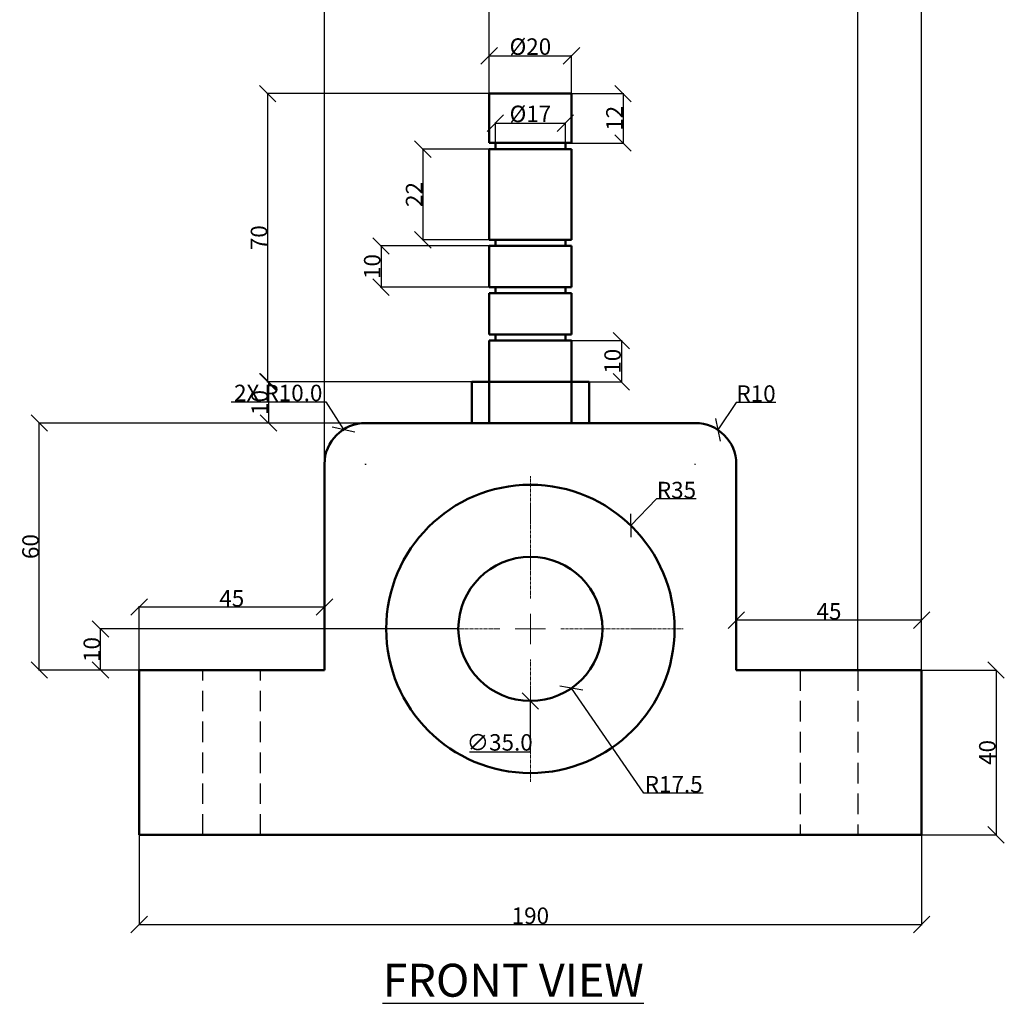
# Model space of a CAD drawing. Units: millimetres. Extents: x 2623 to 3019, y 2308 to 2699.
# Tile 1 of 3: x 2623 to 2862, y 2308 to 2547. Entities that reach past the tile are written whole.
import ezdxf

# ---------------------------------------------------------------- set-up
doc = ezdxf.new("R2010")
doc.units = ezdxf.units.MM
doc.header["$MEASUREMENT"] = 0
doc.linetypes.add('CENTER2', pattern=[1.125, 0.75, -0.125, 0.125, -0.125])
doc.linetypes.add('HIDDEN', pattern=[0.375, 0.25, -0.125])
for name, color, linetype, lineweight in [('M-CNTR', 1, 'CENTER2', 18), ('M-DIMS', 2, 'Continuous', 25), ('M-HIDN', 8, 'HIDDEN', 25), ('M-OUTL', 7, 'Continuous', 50), ('M-TEXT', 7, 'Continuous', 25)]:
    doc.layers.add(name, color=color, linetype=linetype, lineweight=lineweight)
doc.styles.get("Standard").update_dxf_attribs({"font": 'arial.ttf'})
doc.dimstyles.get("Standard").update_dxf_attribs({"dimtxt": 4, "dimasz": 4, "dimexe": 0.18, "dimexo": 0.0625, "dimgap": 0.09, "dimtad": 1, "dimtoh": 1, "dimdec": 0, "dimzin": 0, "dimdsep": 46, "dimtxsty": 'Standard', "dimblk": 'OBLIQUE', "dimcen": 0.09, "dimclre": 251, "dimadec": 0, "dimazin": 0, "dimtfac": 1, "dimtdec": 0, "dimtofl": 0, "dimtmove": 0, "dimatfit": 3, "dimfxl": 1, "dimtolj": 1, "dimtzin": 0, "dimarcsym": 0})

# ---------------------------------------------------------------- blocks, each defined once
blk = doc.blocks.new('_Oblique')
at = {"color": 0, "linetype": 'ByBlock', "lineweight": -2}
blk.add_line((-0.5, -0.5), (0.5, 0.5), dxfattribs=at)
blk = doc.blocks.new('*D2')
at = {"layer": 'Defpoints', "color": 0, "transparency": 16777216}
for p in [(2652.09, 2349.31), (2842.09, 2349.31), (2842.09, 2327.53)]:
    blk.add_point(p, dxfattribs=at)
at = {"layer": 'M-DIMS', "color": 0, "lineweight": -2, "transparency": 16777216}
for p, q in [((2652.09, 2349.25), (2652.09, 2327.35)), ((2842.09, 2349.25), (2842.09, 2327.35)), ((2652.09, 2327.53), (2842.09, 2327.53))]:
    blk.add_line(p, q, dxfattribs=at)
at = {"layer": 'M-DIMS', "color": 0, "lineweight": -2, "transparency": 16777216, "xscale": 4, "yscale": 4, "zscale": 4, "rotation": 180}
blk.add_blockref('_Oblique', (2652.09, 2327.53), dxfattribs=at)
at = {"layer": 'M-DIMS', "color": 0, "lineweight": -2, "transparency": 16777216, "xscale": 4, "yscale": 4, "zscale": 4}
blk.add_blockref('_Oblique', (2842.09, 2327.53), dxfattribs=at)
at = {"layer": 'M-DIMS', "color": 0, "transparency": 16777216, "insert": (2747.09, 2329.66), "char_height": 4, "attachment_point": 5}
blk.add_mtext('\\A1;190', dxfattribs=at)
blk = doc.blocks.new('*D3')
at = {"layer": 'Defpoints', "color": 0, "transparency": 16777216}
for p in [(2842.09, 2389.31), (2842.09, 2349.31), (2860.16, 2349.31)]:
    blk.add_point(p, dxfattribs=at)
at = {"layer": 'M-DIMS', "color": 0, "lineweight": -2, "transparency": 16777216}
for p, q in [((2842.15, 2389.31), (2860.34, 2389.31)), ((2860.16, 2389.31), (2860.16, 2349.31)), ((2842.15, 2349.31), (2860.34, 2349.31))]:
    blk.add_line(p, q, dxfattribs=at)
at = {"layer": 'M-DIMS', "color": 0, "lineweight": -2, "transparency": 16777216, "xscale": 4, "yscale": 4, "zscale": 4}
for p, rotation in [((2860.16, 2389.31), 90), ((2860.16, 2349.31), 270)]:
    blk.add_blockref('_Oblique', p, dxfattribs=dict(at, rotation=rotation))
at = {"layer": 'M-DIMS', "color": 0, "transparency": 16777216, "insert": (2858.03, 2369.31), "char_height": 4, "attachment_point": 5, "rotation": 90}
blk.add_mtext('\\A1;40', dxfattribs=at)
blk = doc.blocks.new('*D4')
at = {"layer": 'Defpoints', "color": 0, "transparency": 16777216}
for p in [(2797.09, 2401.45), (2797.09, 2389.31), (2842.09, 2389.31)]:
    blk.add_point(p, dxfattribs=at)
at = {"layer": 'M-DIMS', "color": 0, "lineweight": -2, "transparency": 16777216}
for p, q in [((2797.09, 2389.37), (2797.09, 2401.63)), ((2842.09, 2401.45), (2797.09, 2401.45)), ((2842.09, 2389.37), (2842.09, 2401.63))]:
    blk.add_line(p, q, dxfattribs=at)
at = {"layer": 'M-DIMS', "color": 0, "lineweight": -2, "transparency": 16777216, "xscale": 4, "yscale": 4, "zscale": 4, "rotation": 180}
blk.add_blockref('_Oblique', (2797.09, 2401.45), dxfattribs=at)
at = {"layer": 'M-DIMS', "color": 0, "lineweight": -2, "transparency": 16777216, "xscale": 4, "yscale": 4, "zscale": 4}
blk.add_blockref('_Oblique', (2842.09, 2401.45), dxfattribs=at)
at = {"layer": 'M-DIMS', "color": 0, "transparency": 16777216, "insert": (2819.59, 2403.58), "char_height": 4, "attachment_point": 5}
blk.add_mtext('\\A1;45', dxfattribs=at)
blk = doc.blocks.new('*D5')
at = {"layer": 'Defpoints', "color": 0, "transparency": 16777216}
for p in [(2652.09, 2404.62), (2652.09, 2389.31), (2697.09, 2389.31)]:
    blk.add_point(p, dxfattribs=at)
at = {"layer": 'M-DIMS', "color": 0, "lineweight": -2, "transparency": 16777216}
for p, q in [((2652.09, 2389.37), (2652.09, 2404.8)), ((2697.09, 2404.62), (2652.09, 2404.62)), ((2697.09, 2389.37), (2697.09, 2404.8))]:
    blk.add_line(p, q, dxfattribs=at)
at = {"layer": 'M-DIMS', "color": 0, "lineweight": -2, "transparency": 16777216, "xscale": 4, "yscale": 4, "zscale": 4, "rotation": 180}
blk.add_blockref('_Oblique', (2652.09, 2404.62), dxfattribs=at)
at = {"layer": 'M-DIMS', "color": 0, "lineweight": -2, "transparency": 16777216, "xscale": 4, "yscale": 4, "zscale": 4}
blk.add_blockref('_Oblique', (2697.09, 2404.62), dxfattribs=at)
at = {"layer": 'M-DIMS', "color": 0, "transparency": 16777216, "insert": (2674.59, 2406.74), "char_height": 4, "attachment_point": 5}
blk.add_mtext('\\A1;45', dxfattribs=at)
blk = doc.blocks.new('*D6')
at = {"layer": 'Defpoints', "color": 0, "transparency": 16777216}
for p in [(2627.85, 2449.31), (2707.09, 2449.31), (2652.09, 2389.31)]:
    blk.add_point(p, dxfattribs=at)
at = {"layer": 'M-DIMS', "color": 0, "lineweight": -2, "transparency": 16777216}
for p, q in [((2707.03, 2449.31), (2627.67, 2449.31)), ((2627.85, 2389.31), (2627.85, 2449.31)), ((2652.03, 2389.31), (2627.67, 2389.31))]:
    blk.add_line(p, q, dxfattribs=at)
at = {"layer": 'M-DIMS', "color": 0, "lineweight": -2, "transparency": 16777216, "xscale": 4, "yscale": 4, "zscale": 4}
for p, rotation in [((2627.85, 2449.31), 90), ((2627.85, 2389.31), 270)]:
    blk.add_blockref('_Oblique', p, dxfattribs=dict(at, rotation=rotation))
at = {"layer": 'M-DIMS', "color": 0, "transparency": 16777216, "insert": (2625.72, 2419.31), "char_height": 4, "attachment_point": 5, "rotation": 90}
blk.add_mtext('\\A1;60', dxfattribs=at)
blk = doc.blocks.new('*D7')
at = {"layer": 'Defpoints', "color": 0, "transparency": 16777216}
for p in [(2642.73, 2399.31), (2729.59, 2399.31), (2652.09, 2389.31)]:
    blk.add_point(p, dxfattribs=at)
at = {"layer": 'M-DIMS', "color": 0, "lineweight": -2, "transparency": 16777216}
for p, q in [((2729.53, 2399.31), (2642.55, 2399.31)), ((2642.73, 2389.31), (2642.73, 2399.31)), ((2652.03, 2389.31), (2642.55, 2389.31))]:
    blk.add_line(p, q, dxfattribs=at)
at = {"layer": 'M-DIMS', "color": 0, "lineweight": -2, "transparency": 16777216, "xscale": 4, "yscale": 4, "zscale": 4}
for p, rotation in [((2642.73, 2399.31), 90), ((2642.73, 2389.31), 270)]:
    blk.add_blockref('_Oblique', p, dxfattribs=dict(at, rotation=rotation))
at = {"layer": 'M-DIMS', "color": 0, "transparency": 16777216, "insert": (2640.6, 2394.31), "char_height": 4, "attachment_point": 5, "rotation": 90}
blk.add_mtext('\\A1;10', dxfattribs=at)
blk = doc.blocks.new('*D8')
at = {"layer": 'Defpoints', "color": 0, "transparency": 16777216}
for p in [(2732.84, 2459.31), (2683.5, 2449.31), (2707.09, 2449.31)]:
    blk.add_point(p, dxfattribs=at)
at = {"layer": 'M-DIMS', "color": 0, "lineweight": -2, "transparency": 16777216}
for p, q in [((2732.78, 2459.31), (2683.32, 2459.31)), ((2683.5, 2459.31), (2683.5, 2449.31)), ((2707.03, 2449.31), (2683.32, 2449.31))]:
    blk.add_line(p, q, dxfattribs=at)
at = {"layer": 'M-DIMS', "color": 0, "lineweight": -2, "transparency": 16777216, "xscale": 4, "yscale": 4, "zscale": 4}
for p, rotation in [((2683.5, 2459.31), 90), ((2683.5, 2449.31), 270)]:
    blk.add_blockref('_Oblique', p, dxfattribs=dict(at, rotation=rotation))
at = {"layer": 'M-DIMS', "color": 0, "transparency": 16777216, "insert": (2681.37, 2454.31), "char_height": 4, "attachment_point": 5, "rotation": 90}
blk.add_mtext('\\A1;10', dxfattribs=at)
blk = doc.blocks.new('*D9')
at = {"layer": 'Defpoints', "color": 0, "transparency": 16777216}
for p in [(2683.32, 2529.31), (2737.09, 2529.31), (2732.84, 2459.31)]:
    blk.add_point(p, dxfattribs=at)
at = {"layer": 'M-DIMS', "color": 0, "lineweight": -2, "transparency": 16777216}
for p, q in [((2737.03, 2529.31), (2683.14, 2529.31)), ((2683.32, 2459.31), (2683.32, 2529.31)), ((2732.78, 2459.31), (2683.14, 2459.31))]:
    blk.add_line(p, q, dxfattribs=at)
at = {"layer": 'M-DIMS', "color": 0, "lineweight": -2, "transparency": 16777216, "xscale": 4, "yscale": 4, "zscale": 4}
for p, rotation in [((2683.32, 2529.31), 90), ((2683.32, 2459.31), 270)]:
    blk.add_blockref('_Oblique', p, dxfattribs=dict(at, rotation=rotation))
at = {"layer": 'M-DIMS', "color": 0, "transparency": 16777216, "insert": (2681.19, 2494.31), "char_height": 4, "attachment_point": 5, "rotation": 90}
blk.add_mtext('\\A1;70', dxfattribs=at)
blk = doc.blocks.new('*D10')
at = {"layer": 'Defpoints', "color": 0, "transparency": 16777216}
for p in [(2737.09, 2515.81), (2720.96, 2493.81), (2737.09, 2493.81)]:
    blk.add_point(p, dxfattribs=at)
at = {"layer": 'M-DIMS', "color": 0, "lineweight": -2, "transparency": 16777216}
for p, q in [((2737.03, 2515.81), (2720.78, 2515.81)), ((2720.96, 2515.81), (2720.96, 2493.81)), ((2737.03, 2493.81), (2720.78, 2493.81))]:
    blk.add_line(p, q, dxfattribs=at)
at = {"layer": 'M-DIMS', "color": 0, "lineweight": -2, "transparency": 16777216, "xscale": 4, "yscale": 4, "zscale": 4}
for p, rotation in [((2720.96, 2515.81), 90), ((2720.96, 2493.81), 270)]:
    blk.add_blockref('_Oblique', p, dxfattribs=dict(at, rotation=rotation))
at = {"layer": 'M-DIMS', "color": 0, "transparency": 16777216, "insert": (2718.86, 2504.81), "char_height": 4, "attachment_point": 5, "rotation": 90}
blk.add_mtext('\\A1;22', dxfattribs=at)
blk = doc.blocks.new('*D11')
at = {"layer": 'Defpoints', "color": 0, "transparency": 16777216}
for p in [(2737.09, 2492.31), (2710.82, 2482.31), (2737.09, 2482.31)]:
    blk.add_point(p, dxfattribs=at)
at = {"layer": 'M-DIMS', "color": 0, "lineweight": -2, "transparency": 16777216}
for p, q in [((2737.03, 2492.31), (2710.64, 2492.31)), ((2710.82, 2492.31), (2710.82, 2482.31)), ((2737.03, 2482.31), (2710.64, 2482.31))]:
    blk.add_line(p, q, dxfattribs=at)
at = {"layer": 'M-DIMS', "color": 0, "lineweight": -2, "transparency": 16777216, "xscale": 4, "yscale": 4, "zscale": 4}
for p, rotation in [((2710.82, 2492.31), 90), ((2710.82, 2482.31), 270)]:
    blk.add_blockref('_Oblique', p, dxfattribs=dict(at, rotation=rotation))
at = {"layer": 'M-DIMS', "color": 0, "transparency": 16777216, "insert": (2708.69, 2487.31), "char_height": 4, "attachment_point": 5, "rotation": 90}
blk.add_mtext('\\A1;10', dxfattribs=at)
blk = doc.blocks.new('*D12')
at = {"layer": 'Defpoints', "color": 0, "transparency": 16777216}
for p in [(2757.09, 2469.31), (2761.34, 2459.31), (2769.19, 2459.31)]:
    blk.add_point(p, dxfattribs=at)
at = {"layer": 'M-DIMS', "color": 0, "lineweight": -2, "transparency": 16777216}
for p, q in [((2757.15, 2469.31), (2769.37, 2469.31)), ((2769.19, 2469.31), (2769.19, 2459.31)), ((2761.4, 2459.31), (2769.37, 2459.31))]:
    blk.add_line(p, q, dxfattribs=at)
at = {"layer": 'M-DIMS', "color": 0, "lineweight": -2, "transparency": 16777216, "xscale": 4, "yscale": 4, "zscale": 4}
for p, rotation in [((2769.19, 2469.31), 90), ((2769.19, 2459.31), 270)]:
    blk.add_blockref('_Oblique', p, dxfattribs=dict(at, rotation=rotation))
at = {"layer": 'M-DIMS', "color": 0, "transparency": 16777216, "insert": (2767.05, 2464.31), "char_height": 4, "attachment_point": 5, "rotation": 90}
blk.add_mtext('\\A1;10', dxfattribs=at)
blk = doc.blocks.new('*D13')
at = {"layer": 'Defpoints', "color": 0, "transparency": 16777216}
for p in [(2757.09, 2538.48), (2737.09, 2529.31), (2757.09, 2529.31)]:
    blk.add_point(p, dxfattribs=at)
at = {"layer": 'M-DIMS', "color": 0, "lineweight": -2, "transparency": 16777216}
for p, q in [((2737.09, 2529.37), (2737.09, 2538.66)), ((2737.09, 2538.48), (2757.09, 2538.48)), ((2757.09, 2529.37), (2757.09, 2538.66))]:
    blk.add_line(p, q, dxfattribs=at)
at = {"layer": 'M-DIMS', "color": 0, "lineweight": -2, "transparency": 16777216, "xscale": 4, "yscale": 4, "zscale": 4, "rotation": 180}
blk.add_blockref('_Oblique', (2737.09, 2538.48), dxfattribs=at)
at = {"layer": 'M-DIMS', "color": 0, "lineweight": -2, "transparency": 16777216, "xscale": 4, "yscale": 4, "zscale": 4}
blk.add_blockref('_Oblique', (2757.09, 2538.48), dxfattribs=at)
at = {"layer": 'M-DIMS', "color": 0, "transparency": 16777216, "insert": (2747.09, 2540.72), "char_height": 4, "attachment_point": 5}
blk.add_mtext('\\A1;%%C20', dxfattribs=at)
blk = doc.blocks.new('*D14')
at = {"layer": 'Defpoints', "color": 0, "transparency": 16777216}
for p in [(2757.09, 2529.31), (2757.09, 2517.31), (2769.6, 2517.31)]:
    blk.add_point(p, dxfattribs=at)
at = {"layer": 'M-DIMS', "color": 0, "lineweight": -2, "transparency": 16777216}
for p, q in [((2757.15, 2529.31), (2769.78, 2529.31)), ((2769.6, 2529.31), (2769.6, 2517.31)), ((2757.15, 2517.31), (2769.78, 2517.31))]:
    blk.add_line(p, q, dxfattribs=at)
at = {"layer": 'M-DIMS', "color": 0, "lineweight": -2, "transparency": 16777216, "xscale": 4, "yscale": 4, "zscale": 4}
for p, rotation in [((2769.6, 2529.31), 90), ((2769.6, 2517.31), 270)]:
    blk.add_blockref('_Oblique', p, dxfattribs=dict(at, rotation=rotation))
at = {"layer": 'M-DIMS', "color": 0, "transparency": 16777216, "insert": (2767.5, 2523.31), "char_height": 4, "attachment_point": 5, "rotation": 90}
blk.add_mtext('\\A1;12', dxfattribs=at)
blk = doc.blocks.new('*D15')
at = {"layer": 'Defpoints', "color": 0, "transparency": 16777216}
for p in [(2755.59, 2522.13), (2738.59, 2517.31), (2755.59, 2517.31)]:
    blk.add_point(p, dxfattribs=at)
at = {"layer": 'M-DIMS', "color": 0, "lineweight": -2, "transparency": 16777216}
for p, q in [((2738.59, 2517.37), (2738.59, 2522.31)), ((2755.59, 2517.37), (2755.59, 2522.31)), ((2738.59, 2522.13), (2755.59, 2522.13))]:
    blk.add_line(p, q, dxfattribs=at)
at = {"layer": 'M-DIMS', "color": 0, "lineweight": -2, "transparency": 16777216, "xscale": 4, "yscale": 4, "zscale": 4, "rotation": 180}
blk.add_blockref('_Oblique', (2738.59, 2522.13), dxfattribs=at)
at = {"layer": 'M-DIMS', "color": 0, "lineweight": -2, "transparency": 16777216, "xscale": 4, "yscale": 4, "zscale": 4}
blk.add_blockref('_Oblique', (2755.59, 2522.13), dxfattribs=at)
at = {"layer": 'M-DIMS', "color": 0, "transparency": 16777216, "insert": (2747.09, 2524.38), "char_height": 4, "attachment_point": 5}
blk.add_mtext('\\A1;%%C17', dxfattribs=at)
blk = doc.blocks.new('*D16')
at = {"layer": 'Defpoints', "color": 0, "transparency": 16777216}
for p in [(2792.61, 2447.65), (2787.09, 2439.31)]:
    blk.add_point(p, dxfattribs=at)
at = {"layer": 'M-DIMS', "color": 0, "lineweight": -2, "transparency": 16777216}
for p, q in [((2797.02, 2454.32), (2792.61, 2447.65)), ((2806.66, 2454.32), (2797.02, 2454.32)), ((2787, 2439.31), (2787.18, 2439.31)), ((2787.09, 2439.22), (2787.09, 2439.4))]:
    blk.add_line(p, q, dxfattribs=at)
at = {"layer": 'M-DIMS', "color": 0, "lineweight": -2, "transparency": 16777216, "xscale": 4, "yscale": 4, "zscale": 4, "rotation": 236.5140954888947}
blk.add_blockref('_Oblique', (2792.61, 2447.65), dxfattribs=at)
at = {"layer": 'M-DIMS', "color": 0, "transparency": 16777216, "insert": (2801.88, 2456.46), "char_height": 4, "attachment_point": 5}
blk.add_mtext('\\A1;R10', dxfattribs=at)
blk = doc.blocks.new('*U17')
at = {"layer": 'M-CNTR', "color": 0, "transparency": 16777216}
for p, q in [((0, 7.4), (0, 37.12)), ((-37.12, 0), (-7.4, 0)), ((7.4, 0), (37.12, 0)), ((0, -37.12), (0, -7.4))]:
    blk.add_line(p, q, dxfattribs=at)
at = {"layer": 'M-CNTR', "color": 0, "linetype": 'Continuous', "transparency": 16777216}
for p, q in [((0, -3.7), (0, 3.7)), ((-3.7, 0), (3.7, 0))]:
    blk.add_line(p, q, dxfattribs=at)
blk = doc.blocks.new('*D18')
at = {"layer": 'Defpoints', "color": 0, "transparency": 16777216}
for p in [(2771.44, 2424.45), (2747.09, 2399.31)]:
    blk.add_point(p, dxfattribs=at)
at = {"layer": 'M-DIMS', "color": 0, "lineweight": -2, "transparency": 16777216}
for p, q in [((2777.68, 2430.9), (2771.44, 2424.45)), ((2787.35, 2430.9), (2777.68, 2430.9)), ((2747, 2399.31), (2747.18, 2399.31)), ((2747.09, 2399.22), (2747.09, 2399.4))]:
    blk.add_line(p, q, dxfattribs=at)
at = {"layer": 'M-DIMS', "color": 0, "lineweight": -2, "transparency": 16777216, "xscale": 4, "yscale": 4, "zscale": 4, "rotation": 225.9219202477783}
blk.add_blockref('_Oblique', (2771.44, 2424.45), dxfattribs=at)
at = {"layer": 'M-DIMS', "color": 0, "transparency": 16777216, "insert": (2782.56, 2433.03), "char_height": 4, "attachment_point": 5}
blk.add_mtext('\\A1;R35', dxfattribs=at)
blk = doc.blocks.new('*D19')
at = {"layer": 'Defpoints', "color": 0, "transparency": 16777216}
for p in [(2747.09, 2399.31), (2757.05, 2384.92)]:
    blk.add_point(p, dxfattribs=at)
at = {"layer": 'M-DIMS', "color": 0, "lineweight": -2, "transparency": 16777216}
for p, q in [((2747, 2399.31), (2747.18, 2399.31)), ((2747.09, 2399.22), (2747.09, 2399.4)), ((2774.67, 2359.45), (2757.05, 2384.92)), ((2789.01, 2359.45), (2774.67, 2359.45))]:
    blk.add_line(p, q, dxfattribs=at)
at = {"layer": 'M-DIMS', "color": 0, "lineweight": -2, "transparency": 16777216, "xscale": 4, "yscale": 4, "zscale": 4, "rotation": 124.6776972359451}
blk.add_blockref('_Oblique', (2757.05, 2384.92), dxfattribs=at)
at = {"layer": 'M-DIMS', "color": 0, "transparency": 16777216, "insert": (2781.88, 2361.58), "char_height": 4, "attachment_point": 5}
blk.add_mtext('\\A1;R17.5', dxfattribs=at)
blk = doc.blocks.new('SHAFT-GROOVED-END-ELEV')
for p, q in [((0, 60), (20, 60)), ((0, 48), (0, 60)), ((20, 48), (20, 60)), ((0, 48), (20, 48)), ((1.5, 46.5), (1.5, 48)), ((18.5, 46.5), (18.5, 48)), ((0, 46.5), (20, 46.5)), ((0, 24.5), (0, 46.5)), ((20, 24.5), (20, 46.5)), ((0, 24.5), (20, 24.5)), ((1.5, 23), (1.5, 24.5)), ((18.5, 23), (18.5, 24.5)), ((0, 23), (20, 23)), ((0, 13), (0, 23)), ((20, 13), (20, 23)), ((0, 13), (20, 13)), ((1.5, 11.5), (1.5, 13)), ((18.5, 11.5), (18.5, 13)), ((0, 11.5), (20, 11.5)), ((0, 1.5), (0, 11.5)), ((20, 1.5), (20, 11.5)), ((0, 1.5), (20, 1.5)), ((1.5, 0), (1.5, 1.5)), ((18.5, 1.5), (18.5, 0)), ((0, 0), (20, 0))]:
    blk.add_line(p, q)
blk = doc.blocks.new('HOLE-D14-HIDDEN-ELEV')
at = {"ltscale": 20}
for p, q in [((0, 0), (0, 40)), ((14, 0), (14, 40))]:
    blk.add_line(p, q, dxfattribs=at)
blk = doc.blocks.new('*D49')
at = {"layer": 'Defpoints', "color": 0, "transparency": 16777216}
for p in [(2842.09, 2694.64), (2826.59, 2389.31), (2842.09, 2389.31)]:
    blk.add_point(p, dxfattribs=at)
at = {"layer": 'M-DIMS', "color": 251, "lineweight": -2, "transparency": 16777216}
for p, q in [((2826.59, 2389.37), (2826.59, 2694.82)), ((2842.09, 2389.37), (2842.09, 2694.82))]:
    blk.add_line(p, q, dxfattribs=at)
at = {"layer": 'M-DIMS', "color": 0, "lineweight": -2, "transparency": 16777216}
blk.add_line((2826.59, 2694.64), (2842.09, 2694.64), dxfattribs=at)
at = {"layer": 'M-DIMS', "color": 0, "lineweight": -2, "transparency": 16777216, "xscale": 4, "yscale": 4, "zscale": 4, "rotation": 180}
blk.add_blockref('_Oblique', (2826.59, 2694.64), dxfattribs=at)
at = {"layer": 'M-DIMS', "color": 0, "lineweight": -2, "transparency": 16777216, "xscale": 4, "yscale": 4, "zscale": 4}
blk.add_blockref('_Oblique', (2842.09, 2694.64), dxfattribs=at)
at = {"layer": 'M-DIMS', "color": 0, "transparency": 16777216, "insert": (2834.34, 2696.78), "char_height": 4, "attachment_point": 5}
blk.add_mtext('\\A1;15.5', dxfattribs=at)
blk = doc.blocks.new('*D52')
at = {"layer": 'Defpoints', "color": 0, "transparency": 16777216}
for p in [(2737.09, 2694.64), (2737.09, 2529.31), (2697.09, 2439.31)]:
    blk.add_point(p, dxfattribs=at)
at = {"layer": 'M-DIMS', "color": 251, "lineweight": -2, "transparency": 16777216}
for p, q in [((2697.09, 2439.37), (2697.09, 2694.82)), ((2737.09, 2529.37), (2737.09, 2694.82))]:
    blk.add_line(p, q, dxfattribs=at)
at = {"layer": 'M-DIMS', "color": 0, "lineweight": -2, "transparency": 16777216}
blk.add_line((2697.09, 2694.64), (2737.09, 2694.64), dxfattribs=at)
at = {"layer": 'M-DIMS', "color": 0, "lineweight": -2, "transparency": 16777216, "xscale": 4, "yscale": 4, "zscale": 4, "rotation": 180}
blk.add_blockref('_Oblique', (2697.09, 2694.64), dxfattribs=at)
at = {"layer": 'M-DIMS', "color": 0, "lineweight": -2, "transparency": 16777216, "xscale": 4, "yscale": 4, "zscale": 4}
blk.add_blockref('_Oblique', (2737.09, 2694.64), dxfattribs=at)
at = {"layer": 'M-DIMS', "color": 0, "transparency": 16777216, "insert": (2717.09, 2696.78), "char_height": 4, "attachment_point": 5}
blk.add_mtext('\\A1;40.0', dxfattribs=at)
blk = doc.blocks.new('*D53')
at = {"layer": 'Defpoints', "color": 0, "transparency": 16777216}
for p in [(2701.7, 2447.74), (2707.09, 2439.31)]:
    blk.add_point(p, dxfattribs=at)
at = {"layer": 'M-DIMS', "color": 0, "lineweight": -2, "transparency": 16777216}
for p, q in [((2674.43, 2454.47), (2697.39, 2454.47)), ((2697.39, 2454.47), (2701.7, 2447.74))]:
    blk.add_line(p, q, dxfattribs=at)
at = {"layer": 'M-DIMS', "color": 251, "lineweight": -2, "transparency": 16777216}
for p, q in [((2707, 2439.31), (2707.18, 2439.31)), ((2707.09, 2439.22), (2707.09, 2439.4))]:
    blk.add_line(p, q, dxfattribs=at)
at = {"layer": 'M-DIMS', "color": 0, "lineweight": -2, "transparency": 16777216, "xscale": 4, "yscale": 4, "zscale": 4, "rotation": 302.6035179105375}
blk.add_blockref('_Oblique', (2701.7, 2447.74), dxfattribs=at)
at = {"layer": 'M-DIMS', "color": 0, "transparency": 16777216, "insert": (2685.87, 2456.61), "char_height": 4, "attachment_point": 5}
blk.add_mtext('\\A1;2X R10.0', dxfattribs=at)
blk = doc.blocks.new('*D55')
at = {"layer": 'Defpoints', "color": 0, "transparency": 16777216}
for p in [(2747.09, 2416.81), (2747.09, 2381.81)]:
    blk.add_point(p, dxfattribs=at)
at = {"layer": 'M-DIMS', "color": 251, "lineweight": -2, "transparency": 16777216}
for p, q in [((2747, 2399.31), (2747.18, 2399.31)), ((2747.09, 2399.22), (2747.09, 2399.4))]:
    blk.add_line(p, q, dxfattribs=at)
at = {"layer": 'M-DIMS', "color": 0, "lineweight": -2, "transparency": 16777216}
for p, q in [((2747.09, 2369.5), (2747.09, 2381.81)), ((2732.27, 2369.5), (2747.09, 2369.5))]:
    blk.add_line(p, q, dxfattribs=at)
at = {"layer": 'M-DIMS', "color": 0, "lineweight": -2, "transparency": 16777216, "xscale": 4, "yscale": 4, "zscale": 4, "rotation": 89.99541306334213}
blk.add_blockref('_Oblique', (2747.09, 2381.81), dxfattribs=at)
at = {"layer": 'M-DIMS', "color": 0, "transparency": 16777216, "insert": (2739.63, 2371.75), "char_height": 4, "attachment_point": 5}
blk.add_mtext('\\A1;∅35.0', dxfattribs=at)

msp = doc.modelspace()

# ---------------------------------------------------------------- linework, layer by layer
at = {"layer": 'M-OUTL'}
for p, q in [((2737.091, 2449.311), (2737.091, 2469.311)), ((2757.091, 2449.311), (2757.091, 2469.311)), ((2707.091, 2449.311), (2787.091, 2449.311)), ((2697.091, 2389.311), (2697.091, 2439.311)), ((2797.091, 2389.311), (2797.091, 2439.311)), ((2652.091, 2349.311), (2652.091, 2389.311)), ((2652.091, 2389.311), (2697.091, 2389.311)), ((2842.091, 2389.311), (2797.091, 2389.311)), ((2842.091, 2349.311), (2842.091, 2389.311)), ((2652.091, 2349.311), (2842.091, 2349.311))]:
    msp.add_line(p, q, dxfattribs=at)
msp.add_lwpolyline([(2732.841, 2459.311), (2761.341, 2459.311), (2761.341, 2449.311), (2732.841, 2449.311)], close=True, dxfattribs=at)
for radius in [35, 17.5]:
    msp.add_circle((2747.091, 2399.311), radius, dxfattribs=at)
for centre, start, end in [((2707.091, 2439.311), 90, 180), ((2787.091, 2439.311), 0, 90)]:
    msp.add_arc(centre, 10, start, end, dxfattribs=at)

# ---------------------------------------------------------------- block references
at = {"layer": 'M-CNTR'}
msp.add_blockref('*U17', (2747.091, 2399.311), dxfattribs=at)
at = {"layer": 'M-HIDN'}
msp.add_blockref('HOLE-D14-HIDDEN-ELEV', (2667.591, 2349.311), dxfattribs=at)
at = {"layer": 'M-HIDN', "rotation": 180}
msp.add_blockref('HOLE-D14-HIDDEN-ELEV', (2826.592, 2389.311), dxfattribs=at)
at = {"layer": 'M-OUTL'}
msp.add_blockref('SHAFT-GROOVED-END-ELEV', (2737.091, 2469.311), dxfattribs=at)

# ---------------------------------------------------------------- texts
at = {"layer": 'M-TEXT', "insert": (2711.215, 2317.991), "char_height": 8, "attachment_point": 1}
msp.add_mtext_dynamic_manual_height_columns('{\\LFRONT VIEW}', width=72.37298, gutter_width=1, heights=[0], dxfattribs=at)

# ---------------------------------------------------------------- dimensions: what is measured, and where the dimension line sits
at = {"layer": 'M-DIMS'}
for base, p1, p2, override, picture, middle in [((2737.091, 2694.644), (2697.091, 2439.311), (2737.091, 2529.311), {"dimdec": 1, "dimlfac": 1, "dimrnd": 0, "dimzin": 0, "dimdsep": 46, "dimlunit": 2}, '*D52', (2717.091, 2696.776)), ((2842.091, 2694.644), (2826.591, 2389.311), (2842.091, 2389.311), {"dimdec": 1, "dimlfac": 1, "dimrnd": 0, "dimzin": 0, "dimdsep": 46, "dimlunit": 2}, '*D49', (2834.341, 2696.776)), ((2652.091, 2404.617), (2697.091, 2389.311), (2652.091, 2389.311), {"dimclrd": 0, "dimclre": 0, "dimclrt": 0}, '*D5', (2674.591, 2406.742)), ((2797.091, 2401.452), (2842.091, 2389.311), (2797.091, 2389.311), {"dimclrd": 0, "dimclre": 0, "dimclrt": 0}, '*D4', (2819.591, 2403.577)), ((2842.091, 2327.526), (2652.091, 2349.311), (2842.091, 2349.311), {"dimclrd": 0, "dimclre": 0, "dimclrt": 0}, '*D2', (2747.091, 2329.658))]:
    dim = msp.add_linear_dim(base=base, p1=p1, p2=p2, dimstyle='Standard', override=override, dxfattribs=at)
    dim.commit()
    dim.dimension.update_dxf_attribs({"geometry": picture, "text_midpoint": middle})
for base, p1, p2, picture, middle in [((2757.091, 2538.477), (2737.091, 2529.311), (2757.091, 2529.311), '*D13', (2747.091, 2540.721)), ((2755.591, 2522.132), (2738.591, 2517.311), (2755.591, 2517.311), '*D15', (2747.091, 2524.376))]:
    dim = msp.add_linear_dim(base=base, p1=p1, p2=p2, text='%%C<>', dimstyle='Standard', override={"dimclrd": 0, "dimclre": 0, "dimclrt": 0}, dxfattribs=at)
    dim.commit()
    dim.dimension.update_dxf_attribs({"geometry": picture, "text_midpoint": middle})
for base, p1, p2, picture, middle in [((2683.323, 2529.311), (2732.841, 2459.311), (2737.091, 2529.311), '*D9', (2681.191, 2494.311)), ((2769.6, 2517.311), (2757.091, 2529.311), (2757.091, 2517.311), '*D14', (2767.502, 2523.311)), ((2720.963, 2493.811), (2737.091, 2515.811), (2737.091, 2493.811), '*D10', (2718.864, 2504.811)), ((2710.822, 2482.311), (2737.091, 2492.311), (2737.091, 2482.311), '*D11', (2708.69, 2487.311)), ((2769.186, 2459.311), (2757.091, 2469.311), (2761.341, 2459.311), '*D12', (2767.054, 2464.311)), ((2683.503, 2449.311), (2732.841, 2459.311), (2707.091, 2449.311), '*D8', (2681.371, 2454.311)), ((2627.851, 2449.311), (2652.091, 2389.311), (2707.091, 2449.311), '*D6', (2625.718, 2419.311)), ((2642.728, 2399.311), (2652.091, 2389.311), (2729.591, 2399.311), '*D7', (2640.596, 2394.311)), ((2860.159, 2349.311), (2842.091, 2389.311), (2842.091, 2349.311), '*D3', (2858.027, 2369.311))]:
    dim = msp.add_linear_dim(base=base, p1=p1, p2=p2, angle=90, dimstyle='Standard', override={"dimclrd": 0, "dimclre": 0, "dimclrt": 0}, dxfattribs=at)
    dim.commit()
    dim.dimension.update_dxf_attribs({"geometry": picture, "text_midpoint": middle})
dim = msp.add_radius_dim(center=(2707.091, 2439.311), mpoint=(2701.703, 2447.735), text='2X <>', dimstyle='Standard', override={"dimdec": 1, "dimlfac": 1, "dimrnd": 0, "dimzin": 0, "dimdsep": 46, "dimlunit": 2}, dxfattribs=at)
dim.commit()
dim.dimension.update_dxf_attribs({"geometry": '*D53', "text_midpoint": (2685.869, 2456.607)})
dim = msp.add_radius_dim(center=(2787.091, 2439.311), mpoint=(2792.609, 2447.651), dimstyle='Standard', override={"dimclrd": 0, "dimclre": 0, "dimclrt": 0}, dxfattribs=at)
dim.commit()
dim.dimension.update_dxf_attribs({"geometry": '*D16', "text_midpoint": (2801.885, 2456.456)})
for mpoint, override, picture, middle in [((2771.439, 2424.455), {"dimclrd": 0, "dimclre": 0, "dimclrt": 0}, '*D18', (2782.561, 2430.897)), ((2757.048, 2384.919), {"dimdec": 1, "dimclrd": 0, "dimclre": 0, "dimclrt": 0}, '*D19', (2781.883, 2359.451))]:
    dim = msp.add_radius_dim(center=(2747.091, 2399.311), mpoint=mpoint, dimstyle='Standard', override=override, dxfattribs=at)
    dim.commit()
    dim.dimension.update_dxf_attribs({"geometry": picture, "text_midpoint": middle, "dimtype": 164})
dim = msp.add_diameter_dim_2p(p1=(2747.093, 2416.811), p2=(2747.09, 2381.811), dimstyle='Standard', override={"dimdec": 1, "dimlfac": 1, "dimrnd": 0, "dimzin": 0, "dimdsep": 46, "dimlunit": 2}, dxfattribs=at)
dim.commit()
dim.dimension.update_dxf_attribs({"geometry": '*D55', "text_midpoint": (2739.635, 2369.503), "dimtype": 163})

doc.saveas('drawing.dxf')
